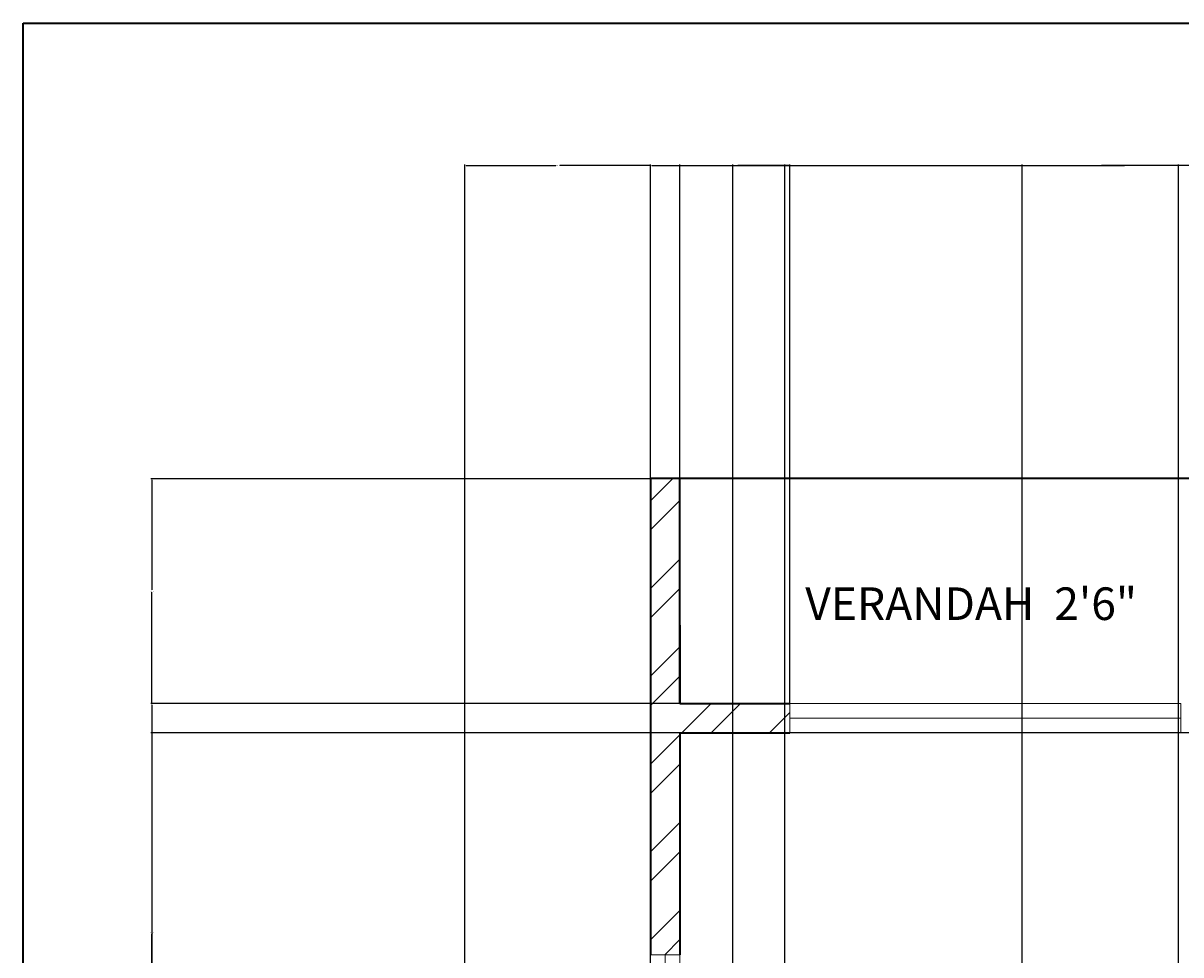
# Model space of a CAD drawing. Units: inches. Extents: x 2008 to 2657, y 1077 to 2165.
# Tile 11 of 16: x 2008 to 2186, y 2022 to 2165. Entities that reach past the tile are written whole.
import ezdxf

# ---------------------------------------------------------------- set-up
doc = ezdxf.new("R2010")
doc.units = ezdxf.units.IN
for name, color, linetype, lineweight in [('A-ANNO-DIMS', 2, 'Continuous', 18), ('A-ANNO-TTLB', 7, 'Continuous', 35), ('A-AREA-IDEN', 4, 'Continuous', 18), ('A-GLAZ', 191, 'Continuous', 18), ('A-WALL', 7, 'Continuous', 35)]:
    doc.layers.add(name, color=color, linetype=linetype, lineweight=lineweight)
doc.layers.add('A-WALL-PATT', color=30, linetype='Continuous', lineweight=13, true_color=0xf8991e)
doc.styles.get("Standard").update_dxf_attribs({"font": 'arial.ttf'})
doc.dimstyles.get("Standard").update_dxf_attribs({"dimtxt": 0.18, "dimasz": 0.18, "dimexe": 0.18, "dimexo": 0.0625, "dimgap": 0.09, "dimtad": 0, "dimtih": 1, "dimtoh": 1, "dimdec": 4, "dimzin": 0, "dimdsep": 46, "dimtxsty": 'Standard', "dimcen": 0.09, "dimadec": 0, "dimazin": 0, "dimtfac": 1, "dimtdec": 4, "dimtofl": 0, "dimtmove": 0, "dimatfit": 3, "dimfxl": 1, "dimtolj": 1, "dimtzin": 0, "dimarcsym": 0})

# ---------------------------------------------------------------- blocks, each defined once
blk = doc.blocks.new('WIN-60IN-B')
for p, q in [((0, 4.5), (0, 0)), ((0, 4.5), (60, 4.5)), ((60, 2.25), (60, 4.5)), ((60, 4.5), (60, 0)), ((0, 0), (0, 2.25)), ((0, 2.25), (60, 2.25)), ((60, 0), (0, 0))]:
    blk.add_line(p, q)
blk = doc.blocks.new('*D33')
at = {"layer": 'A-ANNO-DIMS', "color": 0, "lineweight": -2, "transparency": 16777216}
for p, q in [((2076.26, 1667.3), (2076.26, 2142.9)), ((2104.76, 1667.3), (2104.76, 2142.9)), ((2076.44, 2142.72), (2090.19, 2142.72)), ((2104.58, 2142.72), (2090.84, 2142.72))]:
    blk.add_line(p, q, dxfattribs=at)
at = {"layer": 'A-ANNO-DIMS', "color": 0, "transparency": 16777216}
for points in [[(2076.44, 2142.75), (2076.44, 2142.69), (2076.26, 2142.72)], [(2104.58, 2142.75), (2104.58, 2142.69), (2104.76, 2142.72)]]:
    blk.add_solid(points, dxfattribs=at)
at = {"layer": 'Defpoints', "color": 0, "transparency": 16777216}
for p in [(2104.76, 2142.72), (2076.26, 1667.24), (2104.76, 1667.24)]:
    blk.add_point(p, dxfattribs=at)
at = {"layer": 'A-ANNO-DIMS', "color": 0, "transparency": 16777216, "insert": (2090.51, 2142.72), "char_height": 0.18, "attachment_point": 5}
blk.add_mtext('\\A1;28.5', dxfattribs=at)
blk = doc.blocks.new('*D34')
at = {"layer": 'A-ANNO-DIMS', "color": 0, "lineweight": -2, "transparency": 16777216}
for p, q in [((2104.76, 2094.74), (2104.76, 2142.9)), ((2250.76, 2094.74), (2250.76, 2142.9)), ((2104.94, 2142.72), (2177.48, 2142.72)), ((2250.58, 2142.72), (2178.04, 2142.72))]:
    blk.add_line(p, q, dxfattribs=at)
at = {"layer": 'A-ANNO-DIMS', "color": 0, "transparency": 16777216}
for points in [[(2104.94, 2142.75), (2104.94, 2142.69), (2104.76, 2142.72)], [(2250.58, 2142.75), (2250.58, 2142.69), (2250.76, 2142.72)]]:
    blk.add_solid(points, dxfattribs=at)
at = {"layer": 'Defpoints', "color": 0, "transparency": 16777216}
for p in [(2250.76, 2142.72), (2104.76, 2094.67), (2250.76, 2094.67)]:
    blk.add_point(p, dxfattribs=at)
at = {"layer": 'A-ANNO-DIMS', "color": 0, "transparency": 16777216, "insert": (2177.76, 2142.72), "char_height": 0.18, "attachment_point": 5}
blk.add_mtext('\\A1;146', dxfattribs=at)
blk = doc.blocks.new('*D47')
at = {"layer": 'A-ANNO-DIMS', "color": 0, "lineweight": -2, "transparency": 16777216}
for p, q in [((2109.2, 2060.17), (2028.03, 2060.17)), ((2028.21, 2059.99), (2028.21, 1980.11)), ((2028.21, 1899.85), (2028.21, 1979.74)), ((2109.2, 1899.67), (2028.03, 1899.67))]:
    blk.add_line(p, q, dxfattribs=at)
at = {"layer": 'A-ANNO-DIMS', "color": 0, "transparency": 16777216}
for points in [[(2028.18, 2059.99), (2028.24, 2059.99), (2028.21, 2060.17)], [(2028.18, 1899.85), (2028.24, 1899.85), (2028.21, 1899.67)]]:
    blk.add_solid(points, dxfattribs=at)
at = {"layer": 'Defpoints', "color": 0, "transparency": 16777216}
for p in [(2028.21, 2060.17), (2109.26, 2060.17), (2109.26, 1899.67)]:
    blk.add_point(p, dxfattribs=at)
at = {"layer": 'A-ANNO-DIMS', "color": 0, "transparency": 16777216, "insert": (2028.21, 1979.92), "char_height": 0.18, "attachment_point": 5}
blk.add_mtext('\\A1;160.5', dxfattribs=at)
blk = doc.blocks.new('*D48')
at = {"layer": 'A-ANNO-DIMS', "color": 0, "lineweight": -2, "transparency": 16777216}
for p, q in [((2104.7, 2094.67), (2028.03, 2094.67)), ((2028.21, 2094.49), (2028.21, 2077.61)), ((2028.21, 2060.35), (2028.21, 2077.24)), ((2109.2, 2060.17), (2028.03, 2060.17))]:
    blk.add_line(p, q, dxfattribs=at)
at = {"layer": 'A-ANNO-DIMS', "color": 0, "transparency": 16777216}
for points in [[(2028.18, 2094.49), (2028.24, 2094.49), (2028.21, 2094.67)], [(2028.18, 2060.35), (2028.24, 2060.35), (2028.21, 2060.17)]]:
    blk.add_solid(points, dxfattribs=at)
at = {"layer": 'Defpoints', "color": 0, "transparency": 16777216}
for p in [(2028.21, 2094.67), (2104.76, 2094.67), (2109.26, 2060.17)]:
    blk.add_point(p, dxfattribs=at)
at = {"layer": 'A-ANNO-DIMS', "color": 0, "transparency": 16777216, "insert": (2028.21, 2077.42), "char_height": 0.18, "attachment_point": 5}
blk.add_mtext('\\A1;34.5', dxfattribs=at)
blk = doc.blocks.new('*D54')
at = {"layer": 'A-ANNO-DIMS', "color": 0, "lineweight": -2, "transparency": 16777216}
for p, q in [((2161.76, 1514.3), (2161.76, 2142.9)), ((2185.76, 1514.3), (2185.76, 2142.9)), ((2161.94, 2142.72), (2173.54, 2142.72)), ((2185.58, 2142.72), (2173.98, 2142.72))]:
    blk.add_line(p, q, dxfattribs=at)
at = {"layer": 'A-ANNO-DIMS', "color": 0, "transparency": 16777216}
for points in [[(2161.94, 2142.75), (2161.94, 2142.69), (2161.76, 2142.72)], [(2185.58, 2142.75), (2185.58, 2142.69), (2185.76, 2142.72)]]:
    blk.add_solid(points, dxfattribs=at)
at = {"layer": 'Defpoints', "color": 0, "transparency": 16777216}
for p in [(2185.76, 2142.72), (2161.76, 1514.24), (2185.76, 1514.24)]:
    blk.add_point(p, dxfattribs=at)
at = {"layer": 'A-ANNO-DIMS', "color": 0, "transparency": 16777216, "insert": (2173.76, 2142.72), "char_height": 0.18, "attachment_point": 5}
blk.add_mtext('\\A1;24', dxfattribs=at)
blk = doc.blocks.new('*D61')
at = {"layer": 'A-ANNO-DIMS', "color": 0, "lineweight": -2, "transparency": 16777216}
for p, q in [((2109.26, 2060.24), (2109.26, 2142.9)), ((2126.14, 2060.24), (2126.14, 2142.9)), ((2109.44, 2142.72), (2117.25, 2142.72)), ((2125.96, 2142.72), (2118.16, 2142.72))]:
    blk.add_line(p, q, dxfattribs=at)
at = {"layer": 'A-ANNO-DIMS', "color": 0, "transparency": 16777216}
for points in [[(2109.44, 2142.75), (2109.44, 2142.69), (2109.26, 2142.72)], [(2125.96, 2142.75), (2125.96, 2142.69), (2126.14, 2142.72)]]:
    blk.add_solid(points, dxfattribs=at)
at = {"layer": 'Defpoints', "color": 0, "transparency": 16777216}
for p in [(2126.14, 2142.72), (2109.26, 2060.17), (2126.14, 2060.17)]:
    blk.add_point(p, dxfattribs=at)
at = {"layer": 'A-ANNO-DIMS', "color": 0, "transparency": 16777216, "insert": (2117.7, 2142.72), "char_height": 0.18, "attachment_point": 5}
blk.add_mtext('\\A1;16.877', dxfattribs=at)
blk = doc.blocks.new('*D63')
at = {"layer": 'A-ANNO-DIMS', "color": 0, "lineweight": -2, "transparency": 16777216}
for p, q in [((2117.38, 1662.8), (2117.38, 2142.9)), ((2125.38, 1662.8), (2125.38, 2142.9)), ((2117.56, 2142.72), (2121.23, 2142.72)), ((2125.2, 2142.72), (2121.53, 2142.72))]:
    blk.add_line(p, q, dxfattribs=at)
at = {"layer": 'A-ANNO-DIMS', "color": 0, "transparency": 16777216}
for points in [[(2117.56, 2142.75), (2117.56, 2142.69), (2117.38, 2142.72)], [(2125.2, 2142.75), (2125.2, 2142.69), (2125.38, 2142.72)]]:
    blk.add_solid(points, dxfattribs=at)
at = {"layer": 'Defpoints', "color": 0, "transparency": 16777216}
for p in [(2125.38, 2142.72), (2117.38, 1662.74), (2125.38, 1662.74)]:
    blk.add_point(p, dxfattribs=at)
at = {"layer": 'A-ANNO-DIMS', "color": 0, "transparency": 16777216, "insert": (2121.38, 2142.72), "char_height": 0.18, "attachment_point": 5}
blk.add_mtext('\\A1;8', dxfattribs=at)
blk = doc.blocks.new('*D66')
at = {"layer": 'A-ANNO-DIMS', "color": 0, "lineweight": -2, "transparency": 16777216}
for p, q in [((2572.2, 2055.67), (2028.03, 2055.67)), ((2028.21, 2055.49), (2028.21, 2025.16)), ((2028.21, 1994.47), (2028.21, 2024.8)), ((2572.2, 1994.29), (2028.03, 1994.29))]:
    blk.add_line(p, q, dxfattribs=at)
at = {"layer": 'A-ANNO-DIMS', "color": 0, "transparency": 16777216}
for points in [[(2028.18, 2055.49), (2028.24, 2055.49), (2028.21, 2055.67)], [(2028.18, 1994.47), (2028.24, 1994.47), (2028.21, 1994.29)]]:
    blk.add_solid(points, dxfattribs=at)
at = {"layer": 'Defpoints', "color": 0, "transparency": 16777216}
for p in [(2572.26, 2055.67), (2028.21, 1994.29), (2572.26, 1994.29)]:
    blk.add_point(p, dxfattribs=at)
at = {"layer": 'A-ANNO-DIMS', "color": 0, "transparency": 16777216, "insert": (2028.21, 2024.98), "char_height": 0.18, "attachment_point": 5}
blk.add_mtext('\\A1;61.39', dxfattribs=at)

msp = doc.modelspace()

# ---------------------------------------------------------------- hatches: boundary and pattern name
at = {"layer": 'A-WALL-PATT'}
h = msp.add_hatch(dxfattribs=at)
h.set_pattern_fill('ANSI32', color=256)
h.paths.add_polyline_path([(2109.2619, 2094.6743), (2104.7619, 2094.6743), (2104.7619, 2072.1743), (2104.7619, 2021.6151), (2109.2619, 2021.6151), (2109.2619, 2055.6743), (2126.1387, 2055.6743), (2126.1387, 2057.9243), (2126.1387, 2060.1743), (2109.2619, 2060.1743)])
h.paths.add_polyline_path([(2223.2494, 2057.9243), (2223.2494, 2060.1743), (2186.1387, 2060.1743), (2186.1387, 2055.6743), (2223.2494, 2055.6743)])
h.paths.add_polyline_path([(2250.7619, 2072.1743), (2250.7619, 2090.1743), (2250.7619, 2094.6743), (2246.2619, 2094.6743), (2246.2619, 2060.1743), (2242.7242, 2060.1743), (2242.7242, 2055.6743), (2246.2619, 2055.6743), (2246.2619, 1899.6743), (2242.7458, 1899.6743), (2242.7458, 1897.4243), (2242.7458, 1895.1743), (2246.2619, 1895.1743), (2246.2619, 1878.8745), (2248.5119, 1878.8745), (2250.7619, 1878.8745), (2250.7619, 1991.1743), (2250.7619, 2025.6743), (2257.6798, 2025.6743), (2257.6798, 2027.9243), (2257.6798, 2030.1743), (2250.7619, 2030.1743)])
h.paths.add_polyline_path([(2411.2619, 2031.6743), (2409.0119, 2031.6743), (2406.7619, 2031.6743), (2406.7619, 2030.1743), (2322.7619, 2030.1743), (2322.7619, 2053.3443), (2318.2619, 2053.3443), (2318.2619, 2030.1743), (2305.6798, 2030.1743), (2305.6798, 2025.6743), (2318.2619, 2025.6743), (2322.7619, 2025.6743), (2406.7619, 2025.6743), (2406.7619, 1995.6743), (2406.7619, 1847.2677), (2250.7619, 1847.2677), (2250.7619, 1850.9902), (2248.5119, 1850.9902), (2246.2619, 1850.9902), (2246.2619, 1847.1743), (2246.2619, 1842.7677), (2303.0015, 1842.7677), (2303.0015, 1667.2413), (2298.4208, 1667.2413), (2298.4208, 1662.7413), (2303.0015, 1662.7413), (2303.0015, 1649.8758), (2307.5015, 1649.8758), (2307.5015, 1842.7677), (2406.7619, 1842.7677), (2411.2619, 1842.7677), (2411.2619, 1878.6743), (2415.8196, 1878.6743), (2415.8196, 1880.9243), (2415.8196, 1883.1743), (2411.2619, 1883.1743)])
h.paths.add_polyline_path([(2411.2619, 2094.6743), (2406.7619, 2094.6743), (2318.2619, 2094.6743), (2318.2619, 2077.3443), (2322.7619, 2077.3443), (2322.7619, 2090.1743), (2406.7619, 2090.1743), (2406.7619, 2072.1743), (2406.7619, 2067.6743), (2406.7619, 2052.7524), (2411.2619, 2052.7524), (2411.2619, 2055.6743), (2414.9888, 2055.6743), (2414.9888, 2057.9243), (2414.9888, 2060.1743), (2411.2619, 2060.1743), (2411.2619, 2072.1743)])
h.paths.add_polyline_path([(2576.7619, 2072.1743), (2576.7619, 2094.6743), (2572.2619, 2094.6743), (2572.2619, 2060.1743), (2525.8113, 2060.1743), (2525.8113, 2055.6743), (2572.2619, 2055.6743), (2572.2619, 1994.289), (2576.7619, 1994.289)])
h.paths.add_polyline_path([(2465.8113, 2060.1743), (2436.2802, 2060.1743), (2436.2802, 2055.6743), (2465.8113, 2055.6743), (2465.8113, 2057.9243)])
h.paths.add_polyline_path([(2576.7619, 1934.289), (2574.5119, 1934.289), (2572.2619, 1934.289), (2572.2619, 1883.1743), (2447.7027, 1883.1743), (2447.7027, 1878.6743), (2459.7619, 1878.6743), (2459.7619, 1830.4982), (2464.2619, 1830.4982), (2464.2619, 1878.6743), (2572.2619, 1878.6743), (2572.2619, 1868.4883), (2576.7619, 1868.4883)])
h.paths.add_polyline_path([(2576.7619, 1832.4883), (2572.2619, 1832.4883), (2572.2619, 1806.6743), (2464.2619, 1806.6743), (2464.2619, 1809.6629), (2459.7619, 1809.6629), (2459.7619, 1802.1743), (2483.7619, 1802.1743), (2483.7619, 1778.1743), (2488.2619, 1778.1743), (2488.2619, 1802.1743), (2572.2619, 1802.1743), (2572.2619, 1793.6101), (2576.7619, 1793.6101)])
h.paths.add_polyline_path([(2576.7619, 1769.6101), (2572.2619, 1769.6101), (2572.2619, 1754.1743), (2488.2619, 1754.1743), (2488.2619, 1757.2675), (2486.0119, 1757.2675), (2483.7619, 1757.2675), (2483.7619, 1754.1743), (2447.4528, 1754.1743), (2447.4528, 1749.6743), (2483.7619, 1749.6743), (2572.2619, 1749.6743), (2572.2619, 1715.1837), (2576.7619, 1715.1837)])
h.paths.add_polyline_path([(2576.7619, 1655.1837), (2572.2619, 1655.1837), (2572.2619, 1617.6743), (2411.2619, 1617.6743), (2411.2619, 1749.6743), (2414.2827, 1749.6743), (2414.2827, 1754.1743), (2406.7619, 1754.1743), (2406.7619, 1749.6743), (2406.7619, 1617.6743), (2307.5015, 1617.6743), (2307.5015, 1621.0007), (2305.2515, 1621.0007), (2303.0015, 1621.0007), (2303.0015, 1609.6944), (2307.5015, 1609.6944), (2307.5015, 1613.1743), (2406.7619, 1613.1743), (2406.7619, 1476.6743), (2415.532, 1476.6743), (2415.532, 1478.9243), (2415.532, 1481.1743), (2411.2619, 1481.1743), (2411.2619, 1613.1743), (2572.2619, 1613.1743), (2572.2619, 1584.6086), (2576.7619, 1584.6086)])
h.paths.add_polyline_path([(2576.7619, 1524.6086), (2572.2619, 1524.6086), (2572.2619, 1481.1743), (2483.7619, 1481.1743), (2447.5119, 1481.1743), (2447.5119, 1476.6743), (2483.7619, 1476.6743), (2483.7619, 1473.5051), (2488.2619, 1473.5051), (2488.2619, 1476.6743), (2572.2619, 1476.6743), (2572.2619, 1469.5488), (2576.7619, 1469.5488)])
h.paths.add_polyline_path([(2576.7619, 1445.5488), (2572.2619, 1445.5488), (2572.2619, 1428.6743), (2488.2619, 1428.6743), (2488.2619, 1455.6743), (2486.0119, 1455.6743), (2483.7619, 1455.6743), (2483.7619, 1428.6743), (2459.7619, 1428.6743), (2459.7619, 1422.1519), (2464.2619, 1422.1519), (2464.2619, 1424.1743), (2572.2619, 1424.1743), (2572.2619, 1407.5685), (2576.7619, 1407.5685)])
h.paths.add_polyline_path([(2576.7619, 1371.5685), (2572.2619, 1371.5685), (2572.2619, 1352.1743), (2464.2619, 1352.1743), (2464.2619, 1403.1384), (2462.0119, 1403.1384), (2459.7619, 1403.1384), (2459.7619, 1352.1743), (2446.3194, 1352.1743), (2446.3194, 1347.6743), (2572.2619, 1347.6743), (2572.2619, 1321.0291), (2576.7619, 1321.0291)])
h.paths.add_polyline_path([(2462.703, 1227.6743), (2436.0298, 1227.6743), (2436.0298, 1225.4243), (2436.0298, 1223.1743), (2462.703, 1223.1743), (2462.703, 1225.4243)])
h.paths.add_polyline_path([(2576.7619, 1261.0291), (2574.5119, 1261.0291), (2572.2619, 1261.0291), (2572.2619, 1227.6743), (2522.703, 1227.6743), (2522.703, 1223.1743), (2572.2619, 1223.1743), (2572.2619, 1188.6743), (2576.7619, 1188.6743), (2576.7619, 1193.1743), (2576.7619, 1223.1743)])
h.paths.add_polyline_path([(2414.2823, 1227.6743), (2411.2619, 1227.6743), (2411.2619, 1267.1779), (2409.0119, 1267.1779), (2406.7619, 1267.1779), (2406.7619, 1227.6743), (2322.7619, 1227.6743), (2322.7619, 1244.3623), (2318.2619, 1244.3623), (2318.2619, 1223.1743), (2406.7619, 1223.1743), (2406.7619, 1193.1743), (2406.7619, 1188.6743), (2411.2619, 1188.6743), (2411.2619, 1193.1743), (2411.2619, 1223.1743), (2414.2823, 1223.1743)])
h.paths.add_polyline_path([(2411.2619, 1347.6743), (2414.702, 1347.6743), (2414.702, 1349.9243), (2414.702, 1352.1743), (2411.2619, 1352.1743), (2411.2619, 1416.7413), (2307.5015, 1416.7413), (2307.5015, 1579.8489), (2305.2515, 1579.8489), (2303.0015, 1579.8489), (2303.0015, 1566.7413), (2299.2719, 1566.7413), (2299.2719, 1562.2413), (2303.0015, 1562.2413), (2303.0015, 1416.7413), (2246.2619, 1416.7413), (2246.2619, 1409.8616), (2250.7619, 1409.8616), (2250.7619, 1412.2413), (2406.7619, 1412.2413), (2406.7619, 1292.1743), (2304.9703, 1292.1743), (2304.9703, 1287.6743), (2318.2619, 1287.6743), (2318.2619, 1268.3623), (2322.7619, 1268.3623), (2322.7619, 1287.6743), (2406.7619, 1287.6743), (2406.7619, 1285.4748), (2411.2619, 1285.4748)])
h.paths.add_polyline_path([(2109.2619, 1262.7482), (2104.7619, 1262.7482), (2104.7619, 1223.1743), (2104.7619, 1193.1743), (2104.7619, 1188.6743), (2109.2619, 1188.6743), (2109.2619, 1223.1743), (2126.7928, 1223.1743), (2126.7928, 1225.4243), (2126.7928, 1227.6743), (2109.2619, 1227.6743)])
h.paths.add_polyline_path([(2222.3268, 1227.6743), (2186.7928, 1227.6743), (2186.7928, 1223.1743), (2222.3268, 1223.1743)])
h.paths.add_polyline_path([(2250.7619, 1287.6743), (2256.9703, 1287.6743), (2256.9703, 1289.9243), (2256.9703, 1292.1743), (2250.7619, 1292.1743), (2250.7619, 1382.2078), (2248.5119, 1382.2078), (2246.2619, 1382.2078), (2246.2619, 1347.6743), (2246.2619, 1227.6743), (2242.6068, 1227.6743), (2242.6068, 1223.1743), (2246.2619, 1223.1743), (2246.2619, 1188.6743), (2250.7619, 1188.6743), (2250.7619, 1193.1743), (2250.7619, 1227.6743)])
h.paths.add_polyline_path([(2133.2619, 1349.9243), (2133.2619, 1352.1743), (2109.2619, 1352.1743), (2109.2619, 1375.2826), (2104.7619, 1375.2826), (2104.7619, 1322.7482), (2109.2619, 1322.7482), (2109.2619, 1347.6743), (2133.2619, 1347.6743)])
h.paths.add_polyline_path([(2210.2105, 1352.1743), (2161.7619, 1352.1743), (2161.7619, 1412.2413), (2185.7619, 1412.2413), (2185.7619, 1420.1851), (2183.5119, 1420.1851), (2181.2619, 1420.1851), (2181.2619, 1416.7413), (2109.2619, 1416.7413), (2109.2619, 1452.4006), (2104.7619, 1452.4006), (2104.7619, 1399.2826), (2109.2619, 1399.2826), (2109.2619, 1412.2413), (2157.2619, 1412.2413), (2157.2619, 1352.1743), (2154.3383, 1352.1743), (2154.3383, 1347.6743), (2210.2105, 1347.6743)])
h.paths.add_polyline_path([(2185.7619, 1514.2413), (2161.7619, 1514.2413), (2161.7619, 1518.1307), (2159.5119, 1518.1307), (2157.2619, 1518.1307), (2157.2619, 1514.2413), (2109.2619, 1514.2413), (2109.2619, 1528.997), (2107.0119, 1528.997), (2104.7619, 1528.997), (2104.7619, 1488.4006), (2109.2619, 1488.4006), (2109.2619, 1509.7413), (2181.2619, 1509.7413), (2181.2619, 1441.2042), (2185.7619, 1441.2042)])
h.paths.add_polyline_path([(2270.4025, 1566.7413), (2109.2619, 1566.7413), (2080.7619, 1566.7413), (2080.7619, 1586.5643), (2076.2619, 1586.5643), (2076.2619, 1562.2413), (2080.7619, 1562.2413), (2104.7619, 1562.2413), (2104.7619, 1552.997), (2109.2619, 1552.997), (2109.2619, 1562.2413), (2157.2619, 1562.2413), (2157.2619, 1538.2413), (2161.7619, 1538.2413), (2161.7619, 1562.2413), (2205.2619, 1562.2413), (2270.4025, 1562.2413)])
h.paths.add_polyline_path([(2131.6813, 1897.4243), (2131.6813, 1899.6743), (2109.2619, 1899.6743), (2109.2619, 1961.6151), (2104.7619, 1961.6151), (2104.7619, 1886.8042), (2109.2619, 1886.8042), (2109.2619, 1895.1743), (2131.6813, 1895.1743)])
h.paths.add_polyline_path([(2185.7619, 1847.1743), (2161.7619, 1847.1743), (2161.7619, 1895.1743), (2185.7619, 1895.1743), (2211.543, 1895.1743), (2211.543, 1897.4243), (2211.543, 1899.6743), (2154.0916, 1899.6743), (2154.0916, 1897.4243), (2154.0916, 1895.1743), (2157.2619, 1895.1743), (2157.2619, 1847.1743), (2109.2619, 1847.1743), (2109.2619, 1862.8042), (2104.7619, 1862.8042), (2104.7619, 1821.243), (2109.2619, 1821.243), (2109.2619, 1842.6743), (2181.2619, 1842.6743), (2181.2619, 1840.6763), (2185.7619, 1840.6763)])
h.paths.add_polyline_path([(2109.2619, 1785.243), (2104.7619, 1785.243), (2104.7619, 1715.4691), (2109.2619, 1715.4691), (2109.2619, 1730.8423), (2157.2619, 1730.8423), (2157.2619, 1727.6404), (2161.7619, 1727.6404), (2161.7619, 1730.8423), (2185.7619, 1730.8423), (2185.7619, 1822.1438), (2183.5119, 1822.1438), (2181.2619, 1822.1438), (2181.2619, 1735.3423), (2109.2619, 1735.3423)])
h.paths.add_polyline_path([(2109.2619, 1691.4691), (2104.7619, 1691.4691), (2104.7619, 1667.2413), (2076.2619, 1667.2413), (2076.2619, 1646.5643), (2080.7619, 1646.5643), (2080.7619, 1662.7413), (2109.2619, 1662.7413), (2271.4941, 1662.7413), (2271.4941, 1664.9913), (2271.4941, 1667.2413), (2181.2619, 1667.2413), (2161.7619, 1667.2413), (2161.7619, 1708.3752), (2159.5119, 1708.3752), (2157.2619, 1708.3752), (2157.2619, 1667.2413), (2109.2619, 1667.2413)])
h.paths.add_polyline_path([(2233.1467, 1747.4973), (2270.0737, 1747.4973), (2270.0737, 1766.1547), (2233.1467, 1766.1547)], flags=9)

# ---------------------------------------------------------------- linework, layer by layer
at = {"layer": 'A-ANNO-TTLB'}
msp.add_lwpolyline([(2008.4537, 2164.5615), (2657.4477, 2164.5615), (2657.4477, 1076.8888), (2008.4537, 1076.8888)], close=True, dxfattribs=at)
at = {"layer": 'A-WALL'}
for p, q in [((2250.7619, 2094.6743), (2104.7619, 2094.6743)), ((2104.7619, 2094.6743), (2104.7619, 2072.1743)), ((2109.2619, 2060.1743), (2109.2619, 2094.6743)), ((2104.7619, 2072.1743), (2104.7619, 2021.6151)), ((2109.2619, 2072.1743), (2109.2619, 2060.1743)), ((2109.2619, 2060.1743), (2126.1387, 2060.1743)), ((2109.2619, 2055.6743), (2126.1387, 2055.6743)), ((2109.2619, 2055.6743), (2109.2619, 2021.6151))]:
    msp.add_line(p, q, dxfattribs=at)

# ---------------------------------------------------------------- block references
at = {"layer": 'A-GLAZ'}
msp.add_blockref('WIN-60IN-B', (2126.139, 2055.674), dxfattribs=at)
at = {"layer": 'A-GLAZ', "rotation": 89.99999999999832}
msp.add_blockref('WIN-60IN-B', (2109.2622, 1961.6153), dxfattribs=at)

# ---------------------------------------------------------------- texts
at = {"layer": 'A-AREA-IDEN', "insert": (2128.4927, 2077.9901), "char_height": 5, "attachment_point": 1}
msp.add_mtext_dynamic_manual_height_columns('VERANDAH  2\'6"', width=185.835651, gutter_width=12.5, heights=[0], dxfattribs=at)

# ---------------------------------------------------------------- dimensions: what is measured, and where the dimension line sits
at = {"layer": 'A-ANNO-DIMS'}
for base, p1, p2, override, picture, middle in [((2104.7619, 2142.7243), (2076.2619, 1667.2413), (2104.7619, 1667.2413), {"dimdec": 1, "dimlfac": 1, "dimrnd": 0, "dimzin": 0, "dimdsep": 46, "dimlunit": 2}, '*D33', (2090.5119, 2142.7243)), ((2250.7619, 2142.7243), (2104.7619, 2094.6743), (2250.7619, 2094.6743), {"dimdec": 0, "dimlfac": 1, "dimrnd": 0, "dimzin": 0, "dimdsep": 46, "dimlunit": 2}, '*D34', (2177.7619, 2142.7243)), ((2126.1387, 2142.7243), (2109.2619, 2060.1743), (2126.1387, 2060.1743), {"dimdec": 3, "dimlfac": 1, "dimrnd": 0, "dimzin": 0, "dimdsep": 46, "dimlunit": 2}, '*D61', (2117.7003, 2142.7243)), ((2125.3789, 2142.7243), (2117.3789, 1662.7413), (2125.3789, 1662.7413), {"dimdec": 0, "dimlfac": 1, "dimrnd": 0, "dimzin": 0, "dimdsep": 46, "dimlunit": 2}, '*D63', (2121.3789, 2142.7243)), ((2185.7619, 2142.7243), (2161.7619, 1514.2413), (2185.7619, 1514.2413), {"dimdec": 0, "dimlfac": 1, "dimrnd": 0, "dimzin": 0, "dimdsep": 46, "dimlunit": 2}, '*D54', (2173.7619, 2142.7243))]:
    dim = msp.add_linear_dim(base=base, p1=p1, p2=p2, dimstyle='Standard', override=override, dxfattribs=at)
    dim.commit()
    dim.dimension.update_dxf_attribs({"geometry": picture, "text_midpoint": middle})
for base, p1, p2, override, picture, middle in [((2028.2119, 2094.6743), (2109.2619, 2060.1743), (2104.7619, 2094.6743), {"dimdec": 1, "dimlfac": 1, "dimrnd": 0, "dimzin": 0, "dimdsep": 46, "dimlunit": 2}, '*D48', (2028.2119, 2077.4243)), ((2028.2119, 2060.1743), (2109.2619, 1899.6743), (2109.2619, 2060.1743), {"dimdec": 1, "dimlfac": 1, "dimrnd": 0, "dimzin": 0, "dimdsep": 46, "dimlunit": 2}, '*D47', (2028.2119, 1979.9243)), ((2028.2119, 1994.289), (2572.2619, 2055.6743), (2572.2619, 1994.289), {"dimdec": 2, "dimlfac": 1, "dimrnd": 0, "dimzin": 0, "dimdsep": 46, "dimlunit": 2}, '*D66', (2028.2119, 2024.9817))]:
    dim = msp.add_linear_dim(base=base, p1=p1, p2=p2, angle=90, dimstyle='Standard', override=override, dxfattribs=at)
    dim.commit()
    dim.dimension.update_dxf_attribs({"geometry": picture, "text_midpoint": middle})

doc.saveas('drawing.dxf')
